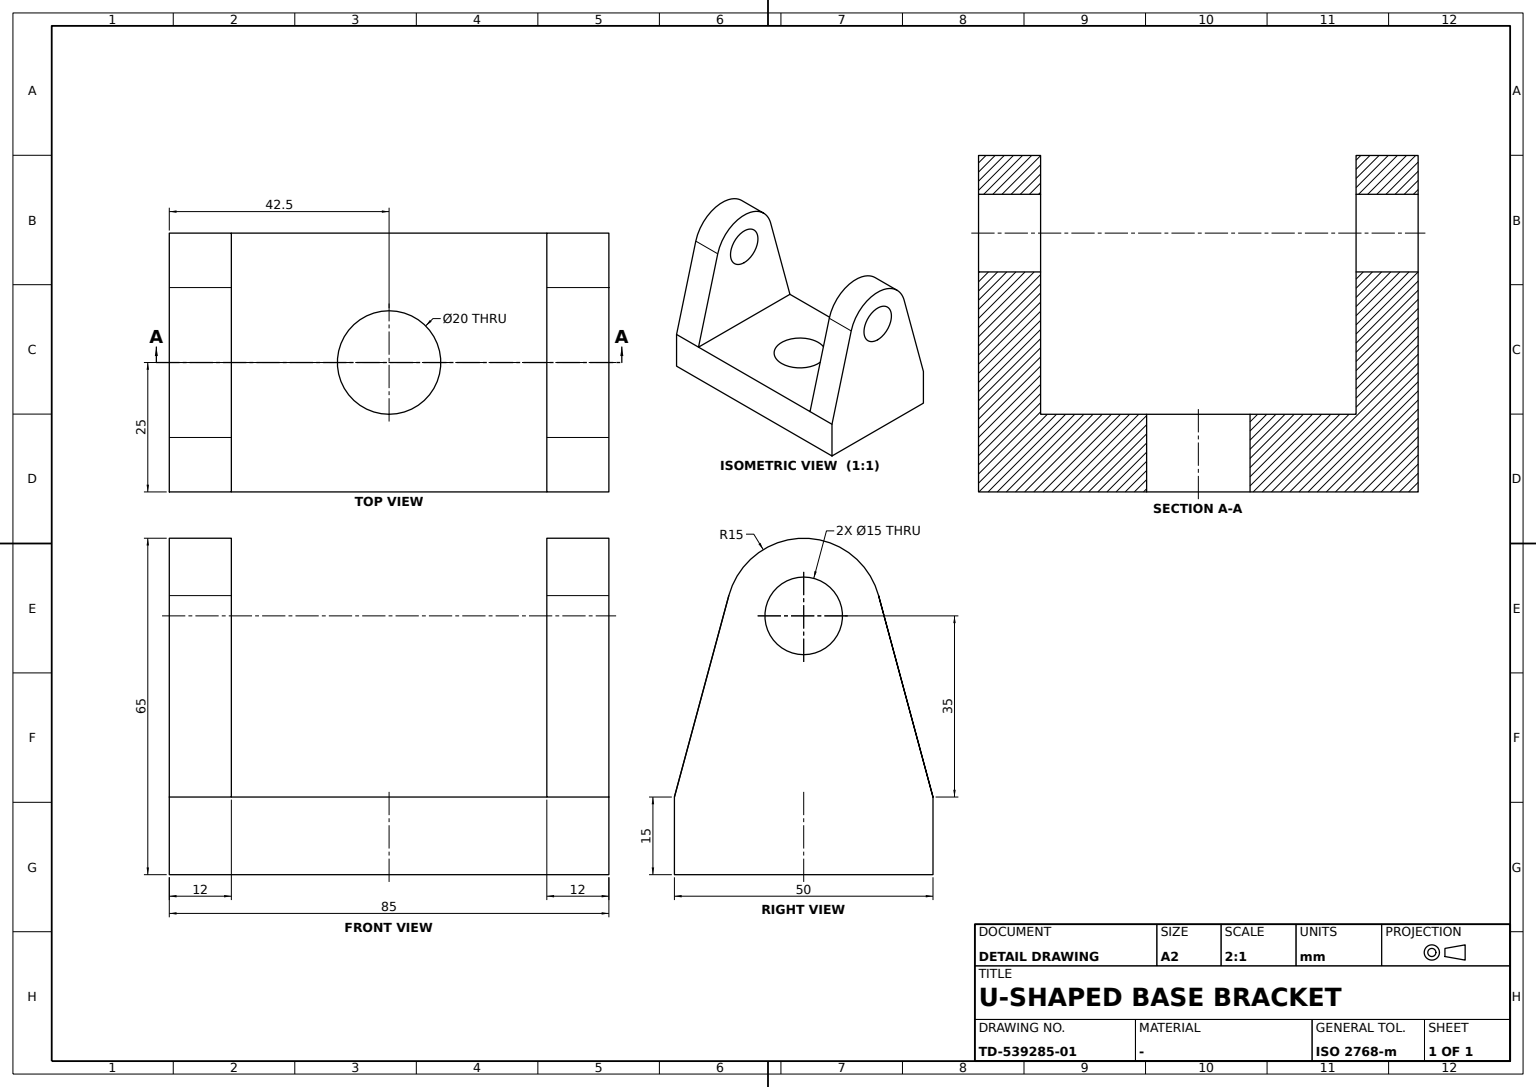
CATIA V5 part; units mm, degrees
sketch "Sketch1" plane through (0, 0, 0) normal (0, 0, 1) x (0, 1, 0)
  line L0 (-42.5, 25) -> (42.5, 25)
  line L1 (42.5, 25) -> (42.5, -25)
  line L2 (42.5, -25) -> (-42.5, -25)
  line L3 (-42.5, -25) -> (-42.5, 25)
  circle A0 centre (0, 0) radius 10
  point P0 (0, -10)
  dimension "length L2" = 85
  dimension "length L1" = 50
  dimension "radius A0" = 10
  constraint horizontal L0 x-axis
  constraint horizontal L2 x-axis
  constraint vertical L1 y-axis
  constraint vertical L3 y-axis
  constraint symmetry L3 L1 y-axis
  constraint symmetry L0 L2 x-axis
  constraint coincidence A0 P0
  constraint coincidence P0 y-axis
extrude "Pad1" add sketch "Sketch1" along normal blind 15
sketch "Sketch2" plane through (0, -42.5, 0) normal (0, -1, 0) x (1, 0, 0)
  arc A0 (14.4802, 53.9145) -> (-14.4802, 53.9145) centre (0, 50) ccw
  point P0 (0, 50)
  point P1 (0, 35)
  circle A1 centre (0, 50) radius 7.5
  point P2 (0, 42.5)
  line L0 (-14.4802, 53.9145) -> (-25, 15)
  line L1 (-25, 15) -> (25, 15)
  point P3 (25, 15)
  line L2 (25, 15) -> (14.4802, 53.9145)
  point P4 (25, 15)
  dimension "radius A0" = 15
  dimension "radius A1" = 7.5
  dimension "distance P0 L1" = 35
  constraint coincidence P0 y-axis
  constraint coincidence A0 P1
  constraint coincidence P1 y-axis
  constraint coincidence A1 P2
  constraint coincidence P2 y-axis
  constraint coincidence P3 P4
  constraint horizontal L1 x-axis
  constraint symmetry L2 L0 y-axis
  constraint tangency L0 A0
extrude "Pad2" add sketch "Sketch2" against normal blind 12
mirror "Mirror1" about plane through (0, 0, 0) normal (0, 1, 0)
